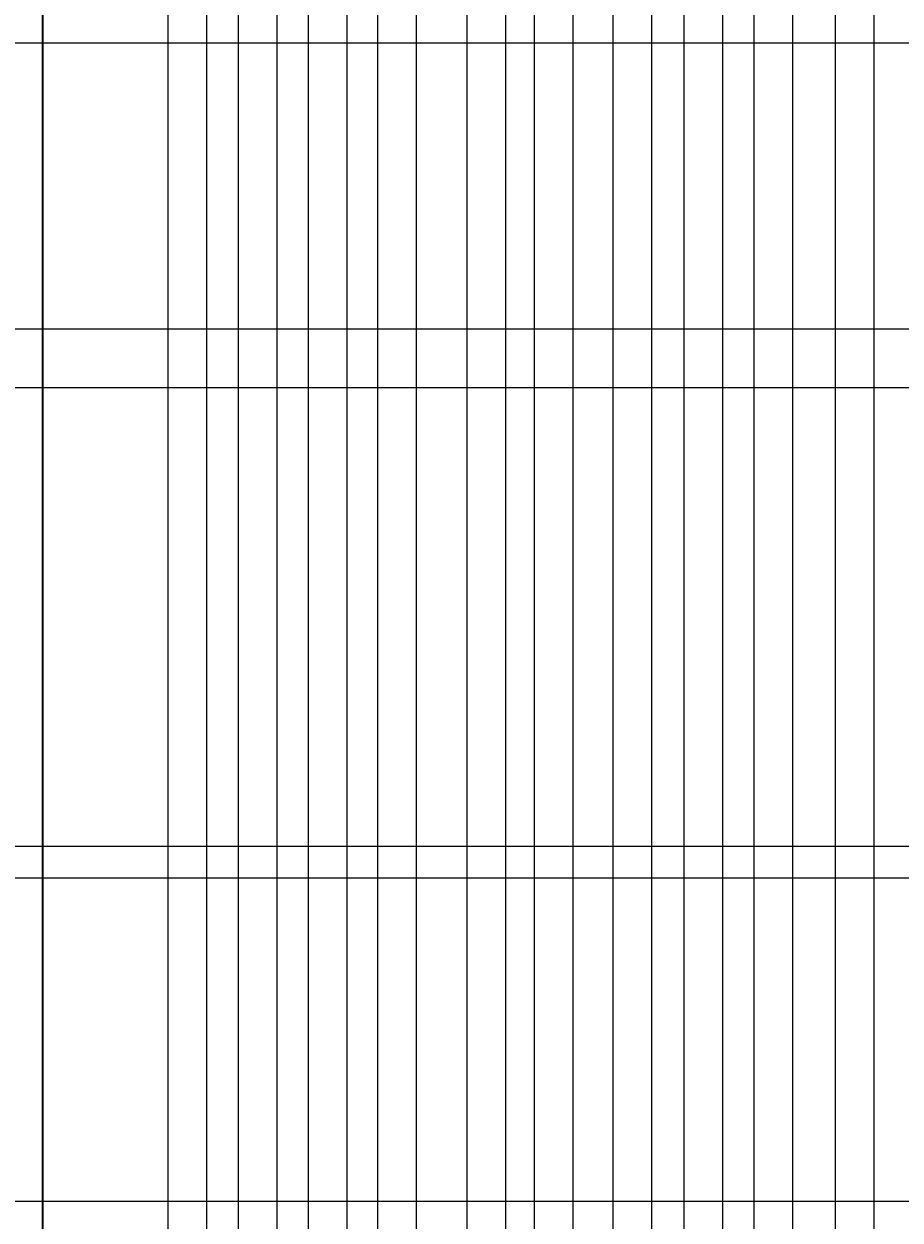
# Model space of a CAD drawing. Units: inches. Extents: x -13 to 809, y 112 to 656.
# Tile 24 of 55: x 339 to 430, y 323 to 446. Entities that reach past the tile are written whole.
import ezdxf

# ---------------------------------------------------------------- set-up
doc = ezdxf.new("R2010")
doc.units = ezdxf.units.IN
doc.header["$MEASUREMENT"] = 0
for name, color, linetype, lineweight in [('A-ANNO-DIMS', 2, 'Continuous', 18), ('A-ELEV', 7, 'Continuous', 35), ('A-ELEV-PATT', 8, 'Continuous', 13)]:
    doc.layers.add(name, color=color, linetype=linetype, lineweight=lineweight)
doc.styles.get("Standard").update_dxf_attribs({"font": 'arial.ttf'})
doc.dimstyles.get("Standard").update_dxf_attribs({"dimtxt": 0.625, "dimasz": 0.18, "dimexe": 0.18, "dimexo": 0.0625, "dimgap": 0.09, "dimtad": 0, "dimtih": 1, "dimtoh": 1, "dimdec": 4, "dimzin": 0, "dimdsep": 46, "dimlunit": 4, "dimtxsty": 'Standard', "dimcen": 0.09, "dimadec": 0, "dimazin": 0, "dimtfac": 1, "dimtdec": 4, "dimtofl": 0, "dimtmove": 0, "dimatfit": 3, "dimfxl": 1, "dimtolj": 1, "dimtzin": 0, "dimarcsym": 0})

# ---------------------------------------------------------------- blocks, each defined once
blk = doc.blocks.new('*D39')
at = {"layer": 'A-ANNO-DIMS', "color": 0, "lineweight": -2, "transparency": 16777216}
for p, q in [((341.34, 524.28), (-12.1, 524.28)), ((-11.92, 524.1), (-11.92, 406.78)), ((-11.92, 288.63), (-11.92, 405.96)), ((341.34, 288.45), (-12.1, 288.45))]:
    blk.add_line(p, q, dxfattribs=at)
at = {"layer": 'A-ANNO-DIMS', "color": 0, "transparency": 16777216}
for points in [[(-11.95, 524.1), (-11.89, 524.1), (-11.92, 524.28)], [(-11.95, 288.63), (-11.89, 288.63), (-11.92, 288.45)]]:
    blk.add_solid(points, dxfattribs=at)
at = {"layer": 'Defpoints', "color": 0, "transparency": 16777216}
for p in [(-11.92, 524.28), (341.41, 524.28), (341.41, 288.45)]:
    blk.add_point(p, dxfattribs=at)
at = {"layer": 'A-ANNO-DIMS', "color": 0, "transparency": 16777216, "insert": (-11.92, 406.37), "char_height": 0.625, "attachment_point": 5}
blk.add_mtext('\\A1;235.83', dxfattribs=at)
blk = doc.blocks.new('*D41')
at = {"layer": 'A-ANNO-DIMS', "color": 0, "lineweight": -2, "transparency": 16777216}
for p, q in [((471.04, 357.98), (-12.1, 357.98)), ((-11.92, 357.8), (-11.92, 335.98)), ((-11.92, 313.35), (-11.92, 335.16)), ((471.04, 313.17), (-12.1, 313.17))]:
    blk.add_line(p, q, dxfattribs=at)
at = {"layer": 'A-ANNO-DIMS', "color": 0, "transparency": 16777216}
for points in [[(-11.95, 357.8), (-11.89, 357.8), (-11.92, 357.98)], [(-11.95, 313.35), (-11.89, 313.35), (-11.92, 313.17)]]:
    blk.add_solid(points, dxfattribs=at)
at = {"layer": 'Defpoints', "color": 0, "transparency": 16777216}
for p in [(-11.92, 357.98), (471.1, 357.98), (471.1, 313.17)]:
    blk.add_point(p, dxfattribs=at)
at = {"layer": 'A-ANNO-DIMS', "color": 0, "transparency": 16777216, "insert": (-11.92, 335.57), "char_height": 0.625, "attachment_point": 5}
blk.add_mtext('\\A1;44.81', dxfattribs=at)
blk = doc.blocks.new('*D42')
at = {"layer": 'A-ANNO-DIMS', "color": 0, "lineweight": -2, "transparency": 16777216}
for p, q in [((471.04, 414.86), (-12.1, 414.86)), ((-11.92, 414.68), (-11.92, 386.83)), ((-11.92, 358.16), (-11.92, 386.01)), ((471.04, 357.98), (-12.1, 357.98))]:
    blk.add_line(p, q, dxfattribs=at)
at = {"layer": 'A-ANNO-DIMS', "color": 0, "transparency": 16777216}
for points in [[(-11.95, 414.68), (-11.89, 414.68), (-11.92, 414.86)], [(-11.95, 358.16), (-11.89, 358.16), (-11.92, 357.98)]]:
    blk.add_solid(points, dxfattribs=at)
at = {"layer": 'Defpoints', "color": 0, "transparency": 16777216}
for p in [(-11.92, 414.86), (471.1, 414.86), (471.1, 357.98)]:
    blk.add_point(p, dxfattribs=at)
at = {"layer": 'A-ANNO-DIMS', "color": 0, "transparency": 16777216, "insert": (-11.92, 386.42), "char_height": 0.625, "attachment_point": 5}
blk.add_mtext('\\A1;56.88', dxfattribs=at)
blk = doc.blocks.new('*D43')
at = {"layer": 'A-ANNO-DIMS', "color": 0, "lineweight": -2, "transparency": 16777216}
for p, q in [((471.04, 470.88), (-12.1, 470.88)), ((-11.92, 470.7), (-11.92, 443.28)), ((-11.92, 415.04), (-11.92, 442.46)), ((471.04, 414.86), (-12.1, 414.86))]:
    blk.add_line(p, q, dxfattribs=at)
at = {"layer": 'A-ANNO-DIMS', "color": 0, "transparency": 16777216}
for points in [[(-11.95, 470.7), (-11.89, 470.7), (-11.92, 470.88)], [(-11.95, 415.04), (-11.89, 415.04), (-11.92, 414.86)]]:
    blk.add_solid(points, dxfattribs=at)
at = {"layer": 'Defpoints', "color": 0, "transparency": 16777216}
for p in [(-11.92, 470.88), (471.1, 470.88), (471.1, 414.86)]:
    blk.add_point(p, dxfattribs=at)
at = {"layer": 'A-ANNO-DIMS', "color": 0, "transparency": 16777216, "insert": (-11.92, 442.87), "char_height": 0.625, "attachment_point": 5}
blk.add_mtext('\\A1;56.02', dxfattribs=at)
blk = doc.blocks.new('*D46')
at = {"layer": 'A-ANNO-DIMS', "color": 0, "lineweight": -2, "transparency": 16777216}
for p, q in [((160.98, 408.79), (807.77, 408.79)), ((807.59, 408.61), (807.59, 367.07)), ((807.59, 324.7), (807.59, 366.25)), ((160.98, 324.52), (807.77, 324.52))]:
    blk.add_line(p, q, dxfattribs=at)
at = {"layer": 'A-ANNO-DIMS', "color": 0, "transparency": 16777216}
for points in [[(807.56, 408.61), (807.62, 408.61), (807.59, 408.79)], [(807.56, 324.7), (807.62, 324.7), (807.59, 324.52)]]:
    blk.add_solid(points, dxfattribs=at)
at = {"layer": 'Defpoints', "color": 0, "transparency": 16777216}
for p in [(160.92, 408.79), (807.59, 408.79), (160.92, 324.52)]:
    blk.add_point(p, dxfattribs=at)
at = {"layer": 'A-ANNO-DIMS', "color": 0, "transparency": 16777216, "insert": (807.59, 366.66), "char_height": 0.625, "attachment_point": 5}
blk.add_mtext('\\A1;84.27', dxfattribs=at)
blk = doc.blocks.new('*D47')
at = {"layer": 'A-ANNO-DIMS', "color": 0, "lineweight": -2, "transparency": 16777216}
for p, q in [((275.78, 408.79), (807.77, 408.79)), ((807.59, 408.61), (807.59, 385.45)), ((807.59, 361.47), (807.59, 384.63)), ((275.78, 361.29), (807.77, 361.29))]:
    blk.add_line(p, q, dxfattribs=at)
at = {"layer": 'A-ANNO-DIMS', "color": 0, "transparency": 16777216}
for points in [[(807.56, 408.61), (807.62, 408.61), (807.59, 408.79)], [(807.56, 361.47), (807.62, 361.47), (807.59, 361.29)]]:
    blk.add_solid(points, dxfattribs=at)
at = {"layer": 'Defpoints', "color": 0, "transparency": 16777216}
for p in [(275.71, 408.79), (807.59, 408.79), (275.71, 361.29)]:
    blk.add_point(p, dxfattribs=at)
at = {"layer": 'A-ANNO-DIMS', "color": 0, "transparency": 16777216, "insert": (807.59, 385.04), "char_height": 0.625, "attachment_point": 5}
blk.add_mtext('\\A1;47.5', dxfattribs=at)
blk = doc.blocks.new('*D48')
at = {"layer": 'A-ANNO-DIMS', "color": 0, "lineweight": -2, "transparency": 16777216}
for p, q in [((319.57, 444.52), (807.77, 444.52)), ((807.59, 444.34), (807.59, 384.93)), ((807.59, 324.7), (807.59, 384.11)), ((319.57, 324.52), (807.77, 324.52))]:
    blk.add_line(p, q, dxfattribs=at)
at = {"layer": 'A-ANNO-DIMS', "color": 0, "transparency": 16777216}
for points in [[(807.56, 444.34), (807.62, 444.34), (807.59, 444.52)], [(807.56, 324.7), (807.62, 324.7), (807.59, 324.52)]]:
    blk.add_solid(points, dxfattribs=at)
at = {"layer": 'Defpoints', "color": 0, "transparency": 16777216}
for p in [(319.51, 444.52), (807.59, 444.52), (319.51, 324.52)]:
    blk.add_point(p, dxfattribs=at)
at = {"layer": 'A-ANNO-DIMS', "color": 0, "transparency": 16777216, "insert": (807.59, 384.52), "char_height": 0.625, "attachment_point": 5}
blk.add_mtext('\\A1;120', dxfattribs=at)
blk = doc.blocks.new('*D105')
at = {"layer": 'A-ANNO-DIMS', "color": 0, "lineweight": -2, "transparency": 16777216}
for p, q in [((319.76, 452.56), (807.77, 452.56)), ((807.59, 452.38), (807.59, 448.95)), ((807.59, 444.7), (807.59, 448.13)), ((319.57, 444.52), (807.77, 444.52))]:
    blk.add_line(p, q, dxfattribs=at)
at = {"layer": 'A-ANNO-DIMS', "color": 0, "transparency": 16777216}
for points in [[(807.56, 452.38), (807.62, 452.38), (807.59, 452.56)], [(807.56, 444.7), (807.62, 444.7), (807.59, 444.52)]]:
    blk.add_solid(points, dxfattribs=at)
at = {"layer": 'Defpoints', "color": 0, "transparency": 16777216}
for p in [(319.7, 452.56), (319.51, 444.52), (807.59, 444.52)]:
    blk.add_point(p, dxfattribs=at)
at = {"layer": 'A-ANNO-DIMS', "color": 0, "transparency": 16777216, "insert": (807.59, 448.54), "char_height": 0.625, "attachment_point": 5}
blk.add_mtext('\\A1;8.043', dxfattribs=at)

msp = doc.modelspace()

# ---------------------------------------------------------------- linework, layer by layer
at = {"layer": 'A-ELEV'}
msp.add_line((341.4072, 210.7849), (341.4072, 524.281), dxfattribs=at)
for points in [[(341.4072, 558.5199), (591.008, 558.5199), (591.008, 250.8429), (341.4072, 250.8429)], [(341.4072, 524.281), (542.9617, 524.281), (542.9617, 288.4508), (341.4072, 288.4508)]]:
    msp.add_lwpolyline(points, close=True, dxfattribs=at)
at = {"layer": 'A-ELEV-PATT'}
for points in [[(354.3886, 288.4508), (354.3886, 523.3908), (354.3886, 524.281)], [(358.3886, 288.4508), (358.3886, 523.3908), (358.3886, 524.281)], [(361.6625, 288.4508), (361.6625, 523.3908), (361.6625, 524.281)], [(365.6625, 288.4508), (365.6625, 523.3908), (365.6625, 524.281)], [(368.9215, 288.4508), (368.9215, 523.3908), (368.9215, 524.281)], [(372.9215, 288.4508), (372.9215, 523.3908), (372.9215, 524.281)], [(376.0866, 288.4508), (376.0866, 523.3908), (376.0866, 524.281)], [(380.0866, 288.4508), (380.0866, 523.3908), (380.0866, 524.281)], [(385.3536, 288.4508), (385.3536, 523.3908), (385.3536, 524.281)], [(389.3536, 288.4508), (389.3536, 523.3908), (389.3536, 524.281)], [(392.3277, 288.4508), (392.3277, 523.3908), (392.3277, 524.281)], [(396.3277, 288.4508), (396.3277, 523.3908), (396.3277, 524.281)], [(400.4483, 288.4508), (400.4483, 523.3908), (400.4483, 524.281)], [(404.4483, 288.4508), (404.4483, 523.3908), (404.4483, 524.281)], [(407.8046, 288.4508), (407.8046, 523.3908), (407.8046, 524.281)], [(411.8046, 288.4508), (411.8046, 523.3908), (411.8046, 524.281)], [(415.0653, 288.4508), (415.0653, 523.3908), (415.0653, 524.281)], [(419.0653, 288.4508), (419.0653, 523.3908), (419.0653, 524.281)], [(423.4725, 288.4508), (423.4725, 523.3908), (423.4725, 524.281)], [(427.4725, 288.4508), (427.4725, 523.3908), (427.4725, 524.281)]]:
    msp.add_lwpolyline(points, dxfattribs=at)

# ---------------------------------------------------------------- dimensions: what is measured, and where the dimension line sits
at = {"layer": 'A-ANNO-DIMS'}
for base, p1, p2, override, picture, middle in [((-11.9191, 524.281), (341.4072, 288.4508), (341.4072, 524.281), {"dimdec": 2, "dimlfac": 1, "dimrnd": 0, "dimzin": 0, "dimdsep": 46, "dimlunit": 2}, '*D39', (-11.9191, 406.3659)), ((-11.9191, 470.8765), (471.0998, 414.8594), (471.0998, 470.8765), {"dimdec": 2, "dimlfac": 1, "dimrnd": 0, "dimzin": 0, "dimdsep": 46, "dimlunit": 2}, '*D43', (-11.9191, 442.8679)), ((807.5888, 444.5199), (319.7004, 452.5629), (319.5074, 444.5199), {"dimdec": 3, "dimlfac": 1, "dimrnd": 0, "dimzin": 0, "dimdsep": 46, "dimlunit": 2}, '*D105', (807.5888, 448.5414)), ((807.5888, 444.5199), (319.5074, 324.5199), (319.5074, 444.5199), {"dimdec": 0, "dimlfac": 1, "dimrnd": 0, "dimzin": 0, "dimdsep": 46, "dimlunit": 2}, '*D48', (807.5888, 384.5199)), ((-11.9191, 414.8594), (471.0998, 357.9804), (471.0998, 414.8594), {"dimdec": 2, "dimlfac": 1, "dimrnd": 0, "dimzin": 0, "dimdsep": 46, "dimlunit": 2}, '*D42', (-11.9191, 386.4199)), ((807.5888, 408.7939), (160.9184, 324.5199), (160.9184, 408.7939), {"dimdec": 2, "dimlfac": 1, "dimrnd": 0, "dimzin": 0, "dimdsep": 46, "dimlunit": 2}, '*D46', (807.5888, 366.6569)), ((807.5888, 408.7939), (275.7145, 361.2915), (275.7145, 408.7939), {"dimdec": 1, "dimlfac": 1, "dimrnd": 0, "dimzin": 0, "dimdsep": 46, "dimlunit": 2}, '*D47', (807.5888, 385.0427)), ((-11.9191, 357.9804), (471.0998, 313.1667), (471.0998, 357.9804), {"dimdec": 2, "dimlfac": 1, "dimrnd": 0, "dimzin": 0, "dimdsep": 46, "dimlunit": 2}, '*D41', (-11.9191, 335.5735))]:
    dim = msp.add_linear_dim(base=base, p1=p1, p2=p2, angle=90, dimstyle='Standard', override=override, dxfattribs=at)
    dim.commit()
    dim.dimension.update_dxf_attribs({"geometry": picture, "text_midpoint": middle})

doc.saveas('drawing.dxf')
